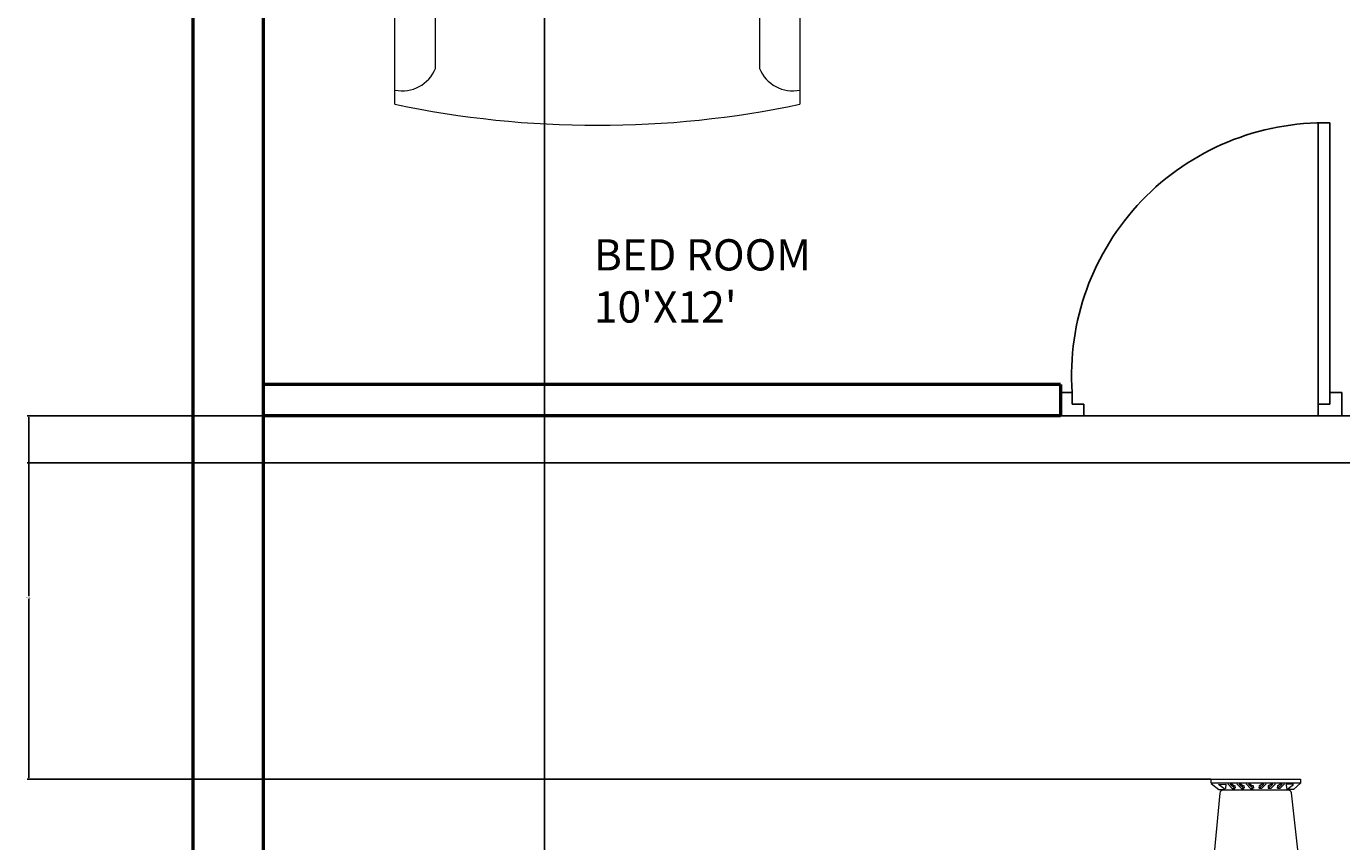
# Model space of a CAD drawing. Units: inches. Extents: x 1798 to 2141, y 1923 to 2386.
# Tile 5 of 9: x 1798 to 1967, y 2177 to 2281. Entities that reach past the tile are written whole.
import ezdxf

# ---------------------------------------------------------------- set-up
doc = ezdxf.new("R2010")
doc.units = ezdxf.units.IN
for name, color, linetype, lineweight in [('A-ANNO-DIMS', 2, 'Continuous', 18), ('A-AREA-IDEN', 7, 'Continuous', 25), ('A-FURN', 8, 'Continuous', 13), ('door', 40, 'Continuous', 25), ('wall', 4, 'Continuous', 50)]:
    doc.layers.add(name, color=color, linetype=linetype, lineweight=lineweight)
doc.styles.get("Standard").update_dxf_attribs({"font": 'arial.ttf'})
doc.dimstyles.get("Standard").update_dxf_attribs({"dimtxt": 0.18, "dimasz": 0.18, "dimexe": 0.18, "dimexo": 0.0625, "dimgap": 0.09, "dimtad": 0, "dimtih": 1, "dimtoh": 1, "dimdec": 4, "dimzin": 0, "dimdsep": 46, "dimtxsty": 'Standard', "dimcen": 0.09, "dimadec": 0, "dimazin": 0, "dimtfac": 1, "dimtdec": 4, "dimtofl": 0, "dimtmove": 0, "dimatfit": 3, "dimfxl": 1, "dimtolj": 1, "dimtzin": 0, "dimarcsym": 0})

# ---------------------------------------------------------------- blocks, each defined once
blk = doc.blocks.new('A$C4F543DC7')
for p, q in [((0.0134, 3.35, -0.1688), (3.3134, 3.35, -0.1688)), ((0.4634, 3.35, -0.1688), (0.0134, 3.35, -0.1688)), ((0.0134, 2.896, -0.1688), (0.0134, 3.35, -0.1688)), ((0.0134, 3.35, -0.1688), (0.0134, 2.896, -0.1688)), ((0.2381, 3.1233, -0.4388), (0.2381, 3.3614, -0.4388)), ((0.4634, 3.35, -0.1688), (0.4634, 0.8, -0.1688)), ((2.8634, 3.35, -0.1688), (0.4634, 3.35, -0.1688)), ((0.4634, 2.896, -0.1688), (0.4634, 3.35, -0.1688)), ((2.8634, 0.8, -0.1688), (2.8634, 3.35, -0.1688)), ((2.8634, 3.35, -0.1688), (3.3134, 3.35, -0.1688)), ((2.8634, 2.896, -0.1688), (2.8634, 3.35, -0.1688)), ((3.0888, 3.1233, -0.4388), (3.0888, 3.3614, -0.4388)), ((3.3134, 3.35, -0.1688), (3.3134, 2.896, -0.1688)), ((3.3134, 3.35, -0.1688), (3.3134, 2.896, -0.1688)), ((1.5354, 3.226, -0.1688), (0.6684, 3.226, -0.1688)), ((2.6644, 3.226, -0.1688), (1.7974, 3.226, -0.1688)), ((0.2381, 3.1233, -0.4388), (0, 3.1233, -0.4388)), ((0.2381, 3.1233, -0.4388), (0.4762, 3.1233, -0.4388)), ((0.2381, 3.1233, -0.4388), (0.2381, 2.8852, -0.4388)), ((0.5684, 3.126, -0.1688), (0.5684, 2.884, -0.1688)), ((1.6354, 2.884, -0.1688), (1.6354, 3.126, -0.1688)), ((1.6974, 3.126, -0.1688), (1.6974, 2.884, -0.1688)), ((2.7644, 2.884, -0.1688), (2.7644, 3.126, -0.1688)), ((3.0888, 3.1233, -0.4388), (2.8507, 3.1233, -0.4388)), ((3.0888, 3.1233, -0.4388), (3.0888, 2.8852, -0.4388)), ((3.0888, 3.1233, -0.4388), (3.3269, 3.1233, -0.4388)), ((0.4634, 2.896, -0.1688), (0.0134, 2.896, -0.1688)), ((0.0134, 2.896, -0.1688), (0.4634, 2.896, -0.1688)), ((0.4634, 0.8, -0.1688), (0.4634, 2.896, -0.1688)), ((2.8634, 2.896, -0.1688), (2.8634, 0.8, -0.1688)), ((3.3134, 2.896, -0.1688), (2.8634, 2.896, -0.1688)), ((3.3134, 2.896, -0.1688), (2.8634, 2.896, -0.1688)), ((0.6684, 2.784, -0.1688), (1.5354, 2.784, -0.1688)), ((1.7974, 2.784, -0.1688), (2.6644, 2.784, -0.1688)), ((1.6534, 2.573, -0.1688), (0.5504, 2.025, -0.1688)), ((0.8414, 1.752, -0.1688), (1.6534, 2.573, -0.1688)), ((2.4814, 1.752, -0.1688), (1.6694, 2.573, -0.1688)), ((1.6694, 2.573, -0.1688), (2.7724, 2.025, -0.1688)), ((0.5504, 2.025, -0.1688), (0.8414, 1.752, -0.1688)), ((2.7724, 2.025, -0.1688), (2.4814, 1.752, -0.1688)), ((2.683, 1.312, -0.1688), (2.7182, 1.3641, -0.1688)), ((0.5369, 1.3267, -0.1688), (0.6088, 1.2835, -0.1688)), ((2.6479, 1.2774, -0.1688), (2.683, 1.312, -0.1688)), ((0.6088, 1.2835, -0.1688), (0.6756, 1.2566, -0.1688)), ((0.6756, 1.2566, -0.1688), (0.7373, 1.2428, -0.1688)), ((0.7373, 1.2428, -0.1688), (0.794, 1.239, -0.1688)), ((0.794, 1.239, -0.1688), (0.8457, 1.242, -0.1688)), ((0.8457, 1.242, -0.1688), (0.8925, 1.2489, -0.1688)), ((0.8925, 1.2489, -0.1688), (0.9345, 1.2564, -0.1688)), ((0.9345, 1.2564, -0.1688), (0.9718, 1.2615, -0.1688)), ((0.9718, 1.2615, -0.1688), (1.0044, 1.2617, -0.1688)), ((1.0044, 1.2617, -0.1688), (1.0334, 1.2578, -0.1688)), ((1.0334, 1.2578, -0.1688), (1.0597, 1.2509, -0.1688)), ((1.0597, 1.2509, -0.1688), (1.0842, 1.2424, -0.1688)), ((1.0842, 1.2424, -0.1688), (1.1081, 1.2336, -0.1688)), ((1.2498, 1.2264, -0.1688), (1.2852, 1.2347, -0.1688)), ((1.2852, 1.2347, -0.1688), (1.3218, 1.2441, -0.1688)), ((1.3218, 1.2441, -0.1688), (1.3591, 1.2533, -0.1688)), ((1.3591, 1.2533, -0.1688), (1.3963, 1.2612, -0.1688)), ((1.3963, 1.2612, -0.1688), (1.4328, 1.2664, -0.1688)), ((1.4328, 1.2664, -0.1688), (1.4679, 1.2677, -0.1688)), ((1.4679, 1.2677, -0.1688), (1.501, 1.2643, -0.1688)), ((1.501, 1.2643, -0.1688), (1.5324, 1.257, -0.1688)), ((1.5324, 1.257, -0.1688), (1.5624, 1.2473, -0.1688)), ((1.5624, 1.2473, -0.1688), (1.5915, 1.2365, -0.1688)), ((1.5915, 1.2365, -0.1688), (1.6199, 1.2259, -0.1688)), ((1.7955, 1.2301, -0.1688), (1.8258, 1.2417, -0.1688)), ((1.8258, 1.2417, -0.1688), (1.8557, 1.2531, -0.1688)), ((1.8557, 1.2531, -0.1688), (1.8849, 1.263, -0.1688)), ((1.8849, 1.263, -0.1688), (1.913, 1.2698, -0.1688)), ((1.913, 1.2698, -0.1688), (1.9397, 1.2722, -0.1688)), ((1.9397, 1.2722, -0.1688), (1.9649, 1.2692, -0.1688)), ((1.9649, 1.2692, -0.1688), (1.989, 1.2617, -0.1688)), ((1.989, 1.2617, -0.1688), (2.0124, 1.2512, -0.1688)), ((2.0124, 1.2512, -0.1688), (2.0359, 1.2391, -0.1688)), ((2.0359, 1.2391, -0.1688), (2.0599, 1.2269, -0.1688)), ((2.2791, 1.2279, -0.1688), (2.3173, 1.2378, -0.1688)), ((2.3173, 1.2378, -0.1688), (2.3558, 1.2465, -0.1688)), ((2.3558, 1.2465, -0.1688), (2.3944, 1.2527, -0.1688)), ((2.3944, 1.2527, -0.1688), (2.4325, 1.255, -0.1688)), ((2.4325, 1.255, -0.1688), (2.4698, 1.2529, -0.1688)), ((2.4698, 1.2529, -0.1688), (2.5064, 1.2488, -0.1688)), ((2.5064, 1.2488, -0.1688), (2.5423, 1.2459, -0.1688)), ((2.5423, 1.2459, -0.1688), (2.5777, 1.2476, -0.1688)), ((2.5777, 1.2476, -0.1688), (2.6129, 1.257, -0.1688)), ((2.6129, 1.257, -0.1688), (2.6479, 1.2774, -0.1688)), ((0.6067, 1.1458, -0.1688), (0.6743, 1.1706, -0.1688)), ((0.6743, 1.1706, -0.1688), (0.7364, 1.1825, -0.1688)), ((0.7364, 1.1825, -0.1688), (0.7931, 1.1846, -0.1688)), ((0.7931, 1.1846, -0.1688), (0.8447, 1.1799, -0.1688)), ((0.8447, 1.1799, -0.1688), (0.8913, 1.1716, -0.1688)), ((0.8913, 1.1716, -0.1688), (0.9331, 1.1628, -0.1688)), ((1.0583, 1.1642, -0.1688), (1.0831, 1.172, -0.1688)), ((1.0831, 1.172, -0.1688), (1.1072, 1.18, -0.1688)), ((1.1072, 1.18, -0.1688), (1.1316, 1.1872, -0.1688)), ((1.1081, 1.2336, -0.1688), (1.1322, 1.2257, -0.1688)), ((1.1316, 1.1872, -0.1688), (1.1573, 1.192, -0.1688)), ((1.1322, 1.2257, -0.1688), (1.1577, 1.2201, -0.1688)), ((1.1573, 1.192, -0.1688), (1.1851, 1.1932, -0.1688)), ((1.1577, 1.2201, -0.1688), (1.1855, 1.218, -0.1688)), ((1.1851, 1.1932, -0.1688), (1.2158, 1.1898, -0.1688)), ((1.1855, 1.218, -0.1688), (1.2163, 1.2204, -0.1688)), ((1.2158, 1.1898, -0.1688), (1.2491, 1.1828, -0.1688)), ((1.2163, 1.2204, -0.1688), (1.2498, 1.2264, -0.1688)), ((1.2491, 1.1828, -0.1688), (1.2842, 1.1734, -0.1688)), ((1.2842, 1.1734, -0.1688), (1.3206, 1.1629, -0.1688)), ((1.5903, 1.1619, -0.1688), (1.6191, 1.1716, -0.1688)), ((1.6191, 1.1716, -0.1688), (1.6475, 1.1797, -0.1688)), ((1.6199, 1.2259, -0.1688), (1.6481, 1.2169, -0.1688)), ((1.6475, 1.1797, -0.1688), (1.676, 1.1849, -0.1688)), ((1.6481, 1.2169, -0.1688), (1.6765, 1.2108, -0.1688)), ((1.676, 1.1849, -0.1688), (1.7049, 1.1858, -0.1688)), ((1.6765, 1.2108, -0.1688), (1.7053, 1.209, -0.1688)), ((1.7049, 1.1858, -0.1688), (1.7344, 1.1816, -0.1688)), ((1.7053, 1.209, -0.1688), (1.7349, 1.2124, -0.1688)), ((1.7344, 1.1816, -0.1688), (1.7643, 1.1731, -0.1688)), ((1.7349, 1.2124, -0.1688), (1.7651, 1.2199, -0.1688)), ((1.7643, 1.1731, -0.1688), (1.7944, 1.1619, -0.1688)), ((1.7651, 1.2199, -0.1688), (1.7955, 1.2301, -0.1688)), ((2.0599, 1.2269, -0.1688), (2.0849, 1.216, -0.1688)), ((2.0842, 1.167, -0.1688), (2.1112, 1.1743, -0.1688)), ((2.0849, 1.216, -0.1688), (2.1117, 1.2077, -0.1688)), ((2.1112, 1.1743, -0.1688), (2.1403, 1.1775, -0.1688)), ((2.1117, 1.2077, -0.1688), (2.1407, 1.2037, -0.1688)), ((2.1403, 1.1775, -0.1688), (2.1718, 1.1755, -0.1688)), ((2.1407, 1.2037, -0.1688), (2.1723, 1.2047, -0.1688)), ((2.1718, 1.1755, -0.1688), (2.2056, 1.1691, -0.1688)), ((2.1723, 1.2047, -0.1688), (2.2062, 1.21, -0.1688)), ((2.2062, 1.21, -0.1688), (2.242, 1.2182, -0.1688)), ((2.242, 1.2182, -0.1688), (2.2791, 1.2279, -0.1688)), ((0.5334, 1.105, -0.1688), (0.6067, 1.1458, -0.1688)), ((0.9331, 1.1628, -0.1688), (0.9701, 1.1565, -0.1688)), ((0.9701, 1.1565, -0.1688), (1.0027, 1.1552, -0.1688)), ((1.0027, 1.1552, -0.1688), (1.0318, 1.1582, -0.1688)), ((1.0318, 1.1582, -0.1688), (1.0583, 1.1642, -0.1688)), ((1.3206, 1.1629, -0.1688), (1.3575, 1.1524, -0.1688)), ((1.3575, 1.1524, -0.1688), (1.3945, 1.1434, -0.1688)), ((1.3945, 1.1434, -0.1688), (1.4308, 1.1371, -0.1688)), ((1.4308, 1.1371, -0.1688), (1.4658, 1.1347, -0.1688)), ((1.4658, 1.1347, -0.1688), (1.499, 1.137, -0.1688)), ((1.499, 1.137, -0.1688), (1.5306, 1.1433, -0.1688)), ((1.5306, 1.1433, -0.1688), (1.5609, 1.152, -0.1688)), ((1.5609, 1.152, -0.1688), (1.5903, 1.1619, -0.1688)), ((1.7944, 1.1619, -0.1688), (1.8244, 1.1494, -0.1688)), ((1.8244, 1.1494, -0.1688), (1.8539, 1.137, -0.1688)), ((1.8539, 1.137, -0.1688), (1.8827, 1.1263, -0.1688)), ((1.8827, 1.1263, -0.1688), (1.9106, 1.1186, -0.1688)), ((1.9106, 1.1186, -0.1688), (1.9373, 1.1153, -0.1688)), ((1.9373, 1.1153, -0.1688), (1.9625, 1.1176, -0.1688)), ((1.9625, 1.1176, -0.1688), (1.9868, 1.1243, -0.1688)), ((1.9868, 1.1243, -0.1688), (2.0106, 1.134, -0.1688)), ((2.0106, 1.134, -0.1688), (2.0344, 1.1454, -0.1688)), ((2.0344, 1.1454, -0.1688), (2.0588, 1.1568, -0.1688)), ((2.0588, 1.1568, -0.1688), (2.0842, 1.167, -0.1688)), ((2.2056, 1.1691, -0.1688), (2.2411, 1.1598, -0.1688)), ((2.2411, 1.1598, -0.1688), (2.2779, 1.1489, -0.1688)), ((2.2779, 1.1489, -0.1688), (2.3157, 1.1379, -0.1688)), ((2.3157, 1.1379, -0.1688), (2.354, 1.1279, -0.1688)), ((2.354, 1.1279, -0.1688), (2.3923, 1.1205, -0.1688)), ((2.3923, 1.1205, -0.1688), (2.4304, 1.117, -0.1688)), ((2.4304, 1.117, -0.1688), (2.4677, 1.118, -0.1688)), ((2.4677, 1.118, -0.1688), (2.5043, 1.1209, -0.1688)), ((2.5043, 1.1209, -0.1688), (2.5403, 1.1226, -0.1688)), ((2.5403, 1.1226, -0.1688), (2.5757, 1.1199, -0.1688)), ((2.5757, 1.1199, -0.1688), (2.6106, 1.1094, -0.1688)), ((2.6106, 1.1094, -0.1688), (2.645, 1.0879, -0.1688)), ((2.645, 1.0879, -0.1688), (2.6789, 1.0522, -0.1688)), ((2.6789, 1.0522, -0.1688), (2.7124, 0.999, -0.1688)), ((0.4634, 0.85, -0.1688), (2.8634, 0.85, -0.1688)), ((0.4634, 0.8, -0.1688), (2.8634, 0.8, -0.1688)), ((0.6634, 0.8, -0.1688), (0.4634, 0.8, -0.1688)), ((0.6634, 0.8, -0.1688), (2.6634, 0.8, -0.1688)), ((0.6634, 0.104, -0.1688), (0.6634, 0.8, -0.1688)), ((0.6634, 0.104, -0.1688), (0.6634, 0.8, -0.1688)), ((0.8634, 0.281, -0.1688), (0.8634, 0.8, -0.1688)), ((2.4634, 0.8, -0.1688), (2.4634, 0.281, -0.1688)), ((2.8634, 0.8, -0.1688), (2.6634, 0.8, -0.1688)), ((2.6634, 0.8, -0.1688), (2.6634, 0.104, -0.1688)), ((2.6634, 0.8, -0.1688), (2.6634, 0.104, -0.1688))]:
    blk.add_line(p, q)
for centre, radius in [((0.2381, 3.1233, -0.4388), 0.139), ((3.0888, 3.1233, -0.4388), 0.139), ((0.2381, 3.1233, -0.4388), 0.075), ((3.0888, 3.1233, -0.4388), 0.075)]:
    blk.add_circle(centre, radius)
for centre, radius, start, end in [((0.6684, 3.126, -0.1688), 0.1, 90, 180), ((1.5354, 3.126, -0.1688), 0.1, 0, 90), ((1.7974, 3.126, -0.1688), 0.1, 90, 180), ((2.6644, 3.126, -0.1688), 0.1, 0, 90), ((0.6684, 2.884, -0.1688), 0.1, 180, 270), ((1.5354, 2.884, -0.1688), 0.1, 270, 0), ((1.7974, 2.884, -0.1688), 0.1, 180, 270), ((2.6644, 2.884, -0.1688), 0.1, 270, 0), ((0.6994, 0.3472, -0.1688), 0.1769, 258.2616, 338.03196), ((2.6275, 0.3472, -0.1688), 0.1769, 201.96804, 281.7384), ((1.6634, 4.8597, -0.1688), 4.8597, 258.12517, 281.87483), ((1.6634, 4.8597, -0.1688), 4.8597, 258.12517, 281.87483)]:
    blk.add_arc(centre, radius, start, end)
blk = doc.blocks.new('A$C45501D90')
for p, q in [((-242.2, 1133.5), (224, 1133.5)), ((-242.2, 1112.8), (-242.2, 1133.5)), ((224, 1112.8), (-242.2, 1112.8)), ((-242.2, 1111.2), (-202.3, 1079.2)), ((-203.9, 1106.4), (-165.6, 1108)), ((-168.8, 1080.8), (-203.9, 1106.4)), ((-165.6, 1108), (-167.2, 1085.6)), ((-156, 1109.6), (-132, 1085.6)), ((-119.3, 1085.6), (-143.2, 1108)), ((-143.2, 1108), (-133.6, 1108)), ((-133.6, 1108), (-122.5, 1098.4)), ((-122.5, 1098.4), (-119.3, 1101.6)), ((-119.3, 1101.6), (-117.7, 1087.2)), ((-108.1, 1109.6), (-84.1, 1085.6)), ((-71.4, 1085.6), (-95.3, 1108)), ((-95.3, 1108), (-85.7, 1108)), ((-85.7, 1108), (-74.6, 1098.4)), ((-74.6, 1098.4), (-71.4, 1101.6)), ((-71.4, 1101.6), (-69.8, 1087.2)), ((-60.2, 1109.6), (-36.2, 1085.6)), ((-23.5, 1085.6), (-47.4, 1108)), ((-47.4, 1108), (-37.8, 1108)), ((-37.8, 1108), (-26.7, 1098.4)), ((-26.7, 1098.4), (-23.5, 1101.6)), ((-23.5, 1101.6), (-21.9, 1087.2)), ((8.5, 1101.6), (6.9, 1087.2)), ((8.5, 1085.6), (32.4, 1108)), ((11.6, 1098.4), (8.5, 1101.6)), ((22.8, 1108), (11.6, 1098.4)), ((45.2, 1109.6), (21.2, 1085.6)), ((32.4, 1108), (22.8, 1108)), ((56.3, 1101.6), (54.8, 1087.2)), ((56.3, 1085.6), (80.3, 1108)), ((59.5, 1098.4), (56.3, 1101.6)), ((70.7, 1108), (59.5, 1098.4)), ((93.1, 1109.6), (69.1, 1085.6)), ((80.3, 1108), (70.7, 1108)), ((104.2, 1101.6), (102.6, 1087.2)), ((104.2, 1085.6), (128.2, 1108)), ((107.4, 1098.4), (104.2, 1101.6)), ((118.6, 1108), (107.4, 1098.4)), ((141, 1109.6), (117, 1085.6)), ((128.2, 1108), (118.6, 1108)), ((188.9, 1106.4), (150.5, 1108)), ((150.5, 1108), (152.1, 1085.6)), ((153.7, 1080.8), (188.9, 1106.4)), ((224, 1112.8), (187.3, 1079.2)), ((224, 1133.5), (224, 1112.8)), ((-197.3, 1061.6), (-238.9, 627.6)), ((-202.3, 1079.2), (-168.8, 1080.8)), ((161.8, 1076.1), (-181.4, 1076.1)), ((-132, 1085.6), (-119.3, 1085.6)), ((-84.1, 1085.6), (-71.4, 1085.6)), ((-36.2, 1085.6), (-23.5, 1085.6)), ((21.2, 1085.6), (8.5, 1085.6)), ((69.1, 1085.6), (56.3, 1085.6)), ((117, 1085.6), (104.2, 1085.6)), ((187.3, 1079.2), (153.7, 1080.8)), ((225.2, 627.8), (177.6, 1061.8)), ((-1102.7, 357), (-869.7, 760.7)), ((-869.7, 760.7), (-851.7, 750.4)), ((841.2, 765.3), (833.5, 714.8)), ((842.6, 766.1), (860.5, 776.5)), ((1075.7, 362.4), (842.6, 766.1)), ((860.5, 776.5), (1093.6, 372.8)), ((-851.7, 750.4), (-1084.8, 346.6)), ((-863.7, 716.7), (-884.3, 684.4)), ((-859.2, 673.6), (-863.7, 716.7)), ((-841, 701.8), (-859.2, 673.6)), ((-848.7, 752.3), (-841, 701.8)), ((820.7, 701.7), (424.1, 520.7)), ((833.5, 714.8), (851.7, 686.6)), ((1012.8, 397.9), (841.2, 695.1)), ((851.7, 686.6), (856.2, 729.8)), ((856.2, 729.8), (876.7, 697.4)), ((876.7, 697.4), (856.6, 687.6)), ((882.9, 689.9), (874.2, 657.2)), ((-851, 678.1), (-1022.6, 380.9)), ((-919.4, 623.5), (-924.2, 615.2)), ((-912, 591.6), (-919.4, 623.5)), ((-914.4, 635.4), (-905.6, 602.7)), ((-897.5, 642.2), (-901.9, 641.1)), ((-901.9, 641.1), (-890.2, 632.5)), ((-895.4, 665), (-900.2, 656.7)), ((-900.2, 656.7), (-897.5, 642.2)), ((-888.1, 633.1), (-895.4, 665)), ((-890.4, 676.9), (-881.7, 644.2)), ((-881.7, 644.2), (-888.1, 633.1)), ((-884.3, 684.4), (-864.1, 674.6)), ((-431.1, 509), (-830.8, 684.8)), ((874.2, 657.2), (880.6, 646.1)), ((880.6, 646.1), (887.9, 678)), ((894.4, 654.1), (882.7, 645.5)), ((887.9, 678), (892.7, 669.7)), ((892.7, 669.7), (890, 655.2)), ((890, 655.2), (894.4, 654.1)), ((906.9, 648.4), (898.1, 615.7)), ((904.5, 604.6), (911.9, 636.5)), ((911.9, 636.5), (916.7, 628.2)), ((916.7, 628.2), (914, 613.8)), ((-945.4, 559.3), (-949.8, 558.1)), ((-949.8, 558.1), (-938.1, 549.6)), ((-943.3, 582), (-948.1, 573.8)), ((-948.1, 573.8), (-945.4, 559.3)), ((-936, 550.1), (-943.3, 582)), ((-938.3, 593.9), (-929.6, 561.2)), ((-929.6, 561.2), (-936, 550.1)), ((-921.5, 600.8), (-925.8, 599.6)), ((-925.8, 599.6), (-914.2, 591)), ((-924.2, 615.2), (-921.5, 600.8)), ((-905.6, 602.7), (-912, 591.6)), ((-223, 610.1), (209.4, 610.1)), ((898.1, 615.7), (904.5, 604.6)), ((918.3, 612.6), (906.7, 604)), ((914, 613.8), (918.3, 612.6)), ((930.8, 606.9), (922.1, 574.2)), ((922.1, 574.2), (928.4, 563.1)), ((928.4, 563.1), (935.8, 595.1)), ((942.3, 571.1), (930.6, 562.6)), ((935.8, 595.1), (940.6, 586.8)), ((940.6, 586.8), (937.9, 572.3)), ((937.9, 572.3), (942.3, 571.1)), ((-1002.4, 479.7), (-988.5, 484.6)), ((-991, 502.7), (-958.3, 511.4)), ((-988.5, 484.6), (-989.7, 489)), ((-989.7, 489), (-976.5, 483.2)), ((-951.9, 522.5), (-983.2, 512.9)), ((-983.2, 512.9), (-978.5, 521.2)), ((-978.5, 521.2), (-964.6, 526.1)), ((-964.6, 526.1), (-965.7, 530.5)), ((-965.7, 530.5), (-952.5, 524.7)), ((-958.3, 511.4), (-951.9, 522.5)), ((-639.9, 111.9), (-423.7, 486.4)), ((-5.6, 508.7, 90.8), (0.4, 508.7, 90.8)), ((-5.6, 317.7, 90.8), (-5.6, 508.7, 90.8)), ((0.4, 508.7, 90.8), (0.4, 317.7, 90.8)), ((5.8, 317.7, 90.8), (5.8, 508.7, 90.8)), ((5.8, 508.7, 90.8), (11.8, 508.7, 90.8)), ((11.8, 508.7, 90.8), (11.8, 317.7, 90.8)), ((416.9, 498.2), (633.1, 123.7)), ((950.8, 524.4), (944.4, 535.5)), ((944.4, 535.5), (975.7, 525.9)), ((958.2, 543.5), (945, 537.7)), ((983.5, 515.7), (950.8, 524.4)), ((957.1, 539.1), (958.2, 543.5)), ((970.9, 534.2), (957.1, 539.1)), ((968.4, 494), (999.7, 484.4)), ((974.7, 483), (968.4, 494)), ((982.2, 502), (968.9, 496.2)), ((975.7, 525.9), (970.9, 534.2)), ((1007.4, 474.2), (974.7, 483)), ((981, 497.6), (982.2, 502)), ((994.9, 492.7), (981, 497.6)), ((999.7, 484.4), (994.9, 492.7)), ((-1038.9, 419.7), (-1006.2, 428.5)), ((-999.8, 439.5), (-1031.1, 430)), ((-1031.1, 430), (-1026.3, 438.3)), ((-1026.3, 438.3), (-1012.5, 443.1)), ((-1015, 461.2), (-982.3, 469.9)), ((-1012.5, 443.1), (-1013.6, 447.5)), ((-1013.6, 447.5), (-1000.4, 441.7)), ((-975.9, 481), (-1007.2, 471.4)), ((-1007.2, 471.4), (-1002.4, 479.7)), ((-1006.2, 428.5), (-999.8, 439.5)), ((-982.3, 469.9), (-975.9, 481)), ((998.7, 441.5), (992.3, 452.5)), ((992.3, 452.5), (1023.6, 443)), ((1006.1, 460.5), (992.9, 454.7)), ((1031.4, 432.7), (998.7, 441.5)), ((1005, 456.2), (1006.1, 460.5)), ((1018.8, 451.3), (1005, 456.2)), ((1034.8, 423.6), (1016.3, 411.1)), ((1023.6, 443), (1018.8, 451.3)), ((1052.6, 389.6), (1034.8, 423.6)), ((-1084.8, 346.6), (-1102.7, 357)), ((-1083.4, 345.8), (-1035.8, 364.4)), ((-1060.1, 376.6), (-1042.3, 410.6)), ((-1020.4, 394.3), (-1060.1, 376.6)), ((-1042.3, 410.6), (-1023.8, 398.1)), ((-1035.8, 364.4), (-1020.4, 394.3)), ((-1018, 360), (-663, 106.9)), ((-22.3, 329.1, 90.8), (-22.3, 344.6, 90.8)), ((-22.3, 344.6, 90.8), (-5.6, 344.6, 90.8)), ((0.4, 344.6, 90.8), (5.8, 344.6, 90.8)), ((11.8, 344.6, 90.8), (27.3, 344.6, 90.8)), ((27.3, 344.6, 90.8), (27.3, 329.1, 90.8)), ((656.3, 118.9), (1008.4, 377.1)), ((1028.3, 377.5), (1012.9, 407.3)), ((1012.9, 407.3), (1052.6, 389.6)), ((1075.9, 358.8), (1028.3, 377.5)), ((1093.6, 372.8), (1075.7, 362.4)), ((-430.6, 275.2, 90.8), (-427.6, 280.3, 90.8)), ((-427.6, 280.3, 90.8), (-262.3, 184.9, 90.8)), ((-175.3, 276.1, 90.8), (-104.8, 293.2, 90.8)), ((-103.3, 252.4, 90.8), (-175.3, 276.1, 90.8)), ((-104.8, 293.2, 90.8), (-85.5, 278.4, 90.8)), ((-85.5, 278.4, 90.8), (-52.1, 293.9, 90.8)), ((9.5, 276.1, 90.8), (-59.5, 246.5, 90.8)), ((-52.1, 293.9, 90.8), (9.5, 276.1, 90.8)), ((-5.6, 329.1, 90.8), (-22.3, 329.1, 90.8)), ((0.4, 317.7, 90.8), (-5.6, 317.7, 90.8)), ((5.8, 329.1, 90.8), (0.4, 329.1, 90.8)), ((11.8, 317.7, 90.8), (5.8, 317.7, 90.8)), ((27.3, 329.1, 90.8), (11.8, 329.1, 90.8)), ((134.3, 288, 90.8), (184.3, 235.5, 90.8)), ((149.7, 213.9, 90.8), (134.3, 288, 90.8)), ((-436.3, 265.3, 90.8), (-433.3, 270.5, 90.8)), ((-270.9, 169.9, 90.8), (-436.3, 265.3, 90.8)), ((-433.3, 270.5, 90.8), (-267.9, 175, 90.8)), ((-265.2, 179.7, 90.8), (-430.6, 275.2, 90.8)), ((-285.5, 198.3, 90.8), (-277.8, 211.7, 90.8)), ((-277.8, 211.7, 90.8), (-264.3, 204, 90.8)), ((-59.5, 246.5, 90.8), (-103.3, 252.4, 90.8)), ((166.5, 173, 90.8), (149.7, 213.9, 90.8)), ((184.3, 235.5, 90.8), (181.1, 211.4, 90.8)), ((181.1, 211.4, 90.8), (211.3, 190.3, 90.8)), ((255.2, 161.9, 90.8), (420.6, 257.3, 90.8)), ((423.5, 252.2, 90.8), (258.2, 156.7, 90.8)), ((260.9, 152, 90.8), (426.2, 247.5, 90.8)), ((429.2, 242.3, 90.8), (263.8, 146.9, 90.8)), ((420.6, 257.3, 90.8), (423.5, 252.2, 90.8)), ((426.2, 247.5, 90.8), (429.2, 242.3, 90.8)), ((-302.5, 168.8, 90.8), (-294.2, 183.3, 90.8)), ((-289.1, 161.1, 90.8), (-302.5, 168.8, 90.8)), ((-291.2, 188.5, 90.8), (-288.5, 193.1, 90.8)), ((-280.7, 175.5, 90.8), (-289.1, 161.1, 90.8)), ((-275.1, 185.4, 90.8), (-277.8, 180.7, 90.8)), ((-273.6, 117.6, 90.8), (-227.4, 162.1, 90.8)), ((-264.3, 204, 90.8), (-272.1, 190.5, 90.8)), ((-267.9, 175, 90.8), (-270.9, 169.9, 90.8)), ((-262.3, 184.9, 90.8), (-265.2, 179.7, 90.8)), ((-227.4, 162.1, 90.8), (-236.2, 87.5, 90.8)), ((226.7, 128.1, 90.8), (166.5, 173, 90.8)), ((211.3, 190.3, 90.8), (226.7, 128.1, 90.8)), ((258.2, 156.7, 90.8), (255.2, 161.9, 90.8)), ((256.6, 182, 90.8), (270.1, 189.8, 90.8)), ((265, 167.5, 90.8), (256.6, 182, 90.8)), ((263.8, 146.9, 90.8), (260.9, 152, 90.8)), ((270.7, 157.7, 90.8), (268, 162.4, 90.8)), ((270.1, 189.8, 90.8), (278.4, 175.3, 90.8)), ((281.4, 139.1, 90.8), (273.7, 152.5, 90.8)), ((281.4, 170.1, 90.8), (284.1, 165.5, 90.8)), ((294.9, 146.8, 90.8), (281.4, 139.1, 90.8)), ((287.1, 160.3, 90.8), (294.9, 146.8, 90.8)), ((-319.8, 2.1, 90.8), (-299.3, 71.7, 90.8)), ((-299.3, 71.7, 90.8), (-276.8, 80.9, 90.8)), ((-276.8, 80.9, 90.8), (-273.6, 117.6, 90.8)), ((-236.2, 87.5, 90.8), (-263.2, 52.5, 90.8)), ((-263.2, 52.5, 90.8), (-319.8, 2.1, 90.8)), ((242.9, -24.6, 90.8), (299.4, 25.9, 90.8)), ((299.4, 25.9, 90.8), (278.9, -43.7, 90.8)), ((207, -134.1, 90.8), (215.8, -59.5, 90.8)), ((215.8, -59.5, 90.8), (242.9, -24.6, 90.8)), ((256.4, -53, 90.8), (253.2, -89.7, 90.8)), ((278.9, -43.7, 90.8), (256.4, -53, 90.8)), ((-656.3, -118.9), (-1008.4, -377.1)), ((-416.9, -498.2), (-633.1, -123.7)), ((-449.6, -214.4, 90.8), (-284.2, -118.9, 90.8)), ((-281.2, -124.1, 90.8), (-446.6, -219.5, 90.8)), ((-443.9, -224.2, 90.8), (-278.5, -128.7, 90.8)), ((-275.5, -133.9, 90.8), (-440.9, -229.4, 90.8)), ((-315.2, -118.9, 90.8), (-301.8, -111.1, 90.8)), ((-307.5, -132.3, 90.8), (-315.2, -118.9, 90.8)), ((-301.8, -142.1, 90.8), (-304.5, -137.5, 90.8)), ((-301.8, -111.1, 90.8), (-294, -124.6, 90.8)), ((-291, -129.7, 90.8), (-288.3, -134.4, 90.8)), ((-284.2, -118.9, 90.8), (-281.2, -124.1, 90.8)), ((-278.5, -128.7, 90.8), (-275.5, -133.9, 90.8)), ((-247, -100.1, 90.8), (-186.8, -145, 90.8)), ((-231.7, -162.3, 90.8), (-247, -100.1, 90.8)), ((253.2, -89.7, 90.8), (207, -134.1, 90.8)), ((260.4, -147.6, 90.8), (268.7, -133.1, 90.8)), ((268.7, -133.1, 90.8), (282.2, -140.8, 90.8)), ((639.9, -111.9), (423.7, -486.4)), ((1018, -360), (663, -106.9)), ((-290.4, -161.8, 90.8), (-298.8, -147.3, 90.8)), ((-277, -154, 90.8), (-290.4, -161.8, 90.8)), ((-285.4, -139.5, 90.8), (-277, -154, 90.8)), ((-201.5, -183.4, 90.8), (-231.7, -162.3, 90.8)), ((-204.7, -207.6, 90.8), (-201.5, -183.4, 90.8)), ((-186.8, -145, 90.8), (-170.1, -185.9, 90.8)), ((-170.1, -185.9, 90.8), (-154.7, -260.1, 90.8)), ((241.9, -156.9, 90.8), (244.9, -151.7, 90.8)), ((407.3, -252.4, 90.8), (241.9, -156.9, 90.8)), ((244, -176, 90.8), (251.7, -162.5, 90.8)), ((257.4, -183.7, 90.8), (244, -176, 90.8)), ((244.9, -151.7, 90.8), (410.3, -247.2, 90.8)), ((247.6, -147.1, 90.8), (250.6, -141.9, 90.8)), ((413, -242.5, 90.8), (247.6, -147.1, 90.8)), ((250.6, -141.9, 90.8), (415.9, -237.4, 90.8)), ((254.7, -157.4, 90.8), (257.4, -152.7, 90.8)), ((265.2, -170.3, 90.8), (257.4, -183.7, 90.8)), ((270.8, -160.5, 90.8), (268.1, -165.1, 90.8)), ((282.2, -140.8, 90.8), (273.8, -155.3, 90.8)), ((-446.6, -219.5, 90.8), (-449.6, -214.4, 90.8)), ((-440.9, -229.4, 90.8), (-443.9, -224.2, 90.8)), ((-154.7, -260.1, 90.8), (-204.7, -207.6, 90.8)), ((-29.8, -248.2, 90.8), (39.2, -218.5, 90.8)), ((31.8, -266, 90.8), (-29.8, -248.2, 90.8)), ((65.2, -250.4, 90.8), (31.8, -266, 90.8)), ((39.2, -218.5, 90.8), (83, -224.4, 90.8)), ((84.4, -265.2, 90.8), (65.2, -250.4, 90.8)), ((83, -224.4, 90.8), (154.9, -248.2, 90.8)), ((154.9, -248.2, 90.8), (84.4, -265.2, 90.8)), ((410.3, -247.2, 90.8), (407.3, -252.4, 90.8)), ((415.9, -237.4, 90.8), (413, -242.5, 90.8)), ((-47.6, -316.6, 90.8), (-47.6, -301.1, 90.8)), ((-47.6, -301.1, 90.8), (-32.1, -301.1, 90.8)), ((-32.1, -316.6, 90.8), (-47.6, -316.6, 90.8)), ((-32.1, -480.7, 90.8), (-32.1, -289.8, 90.8)), ((-32.1, -289.8, 90.8), (-26.1, -289.8, 90.8)), ((-26.1, -289.8, 90.8), (-26.1, -480.7, 90.8)), ((-26.1, -301.1, 90.8), (-20.8, -301.1, 90.8)), ((-20.8, -316.6, 90.8), (-26.1, -316.6, 90.8)), ((-20.8, -480.7, 90.8), (-20.8, -289.8, 90.8)), ((-20.8, -289.8, 90.8), (-14.8, -289.8, 90.8)), ((-14.8, -289.8, 90.8), (-14.8, -480.7, 90.8)), ((-14.8, -301.1, 90.8), (1.9, -301.1, 90.8)), ((1.9, -316.6, 90.8), (-14.8, -316.6, 90.8)), ((1.9, -301.1, 90.8), (1.9, -316.6, 90.8)), ((-1093.6, -372.8), (-1075.7, -362.4)), ((-860.5, -776.5), (-1093.6, -372.8)), ((-1075.9, -358.8), (-1028.3, -377.5)), ((-1075.7, -362.4), (-842.6, -766.1)), ((-1052.6, -389.6), (-1034.8, -423.6)), ((-1012.9, -407.3), (-1052.6, -389.6)), ((-1034.8, -423.6), (-1016.3, -411.1)), ((-1028.3, -377.5), (-1012.9, -407.3)), ((-1012.8, -397.9), (-841.2, -695.1)), ((851, -678.1), (1022.6, -380.9)), ((851.7, -750.4), (1084.8, -346.6)), ((1102.7, -357), (869.7, -760.7)), ((1035.8, -364.4), (1020.4, -394.3)), ((1020.4, -394.3), (1060.1, -376.6)), ((1042.3, -410.6), (1023.8, -398.1)), ((1083.4, -345.8), (1035.8, -364.4)), ((1060.1, -376.6), (1042.3, -410.6)), ((1084.8, -346.6), (1102.7, -357)), ((-1031.4, -432.7), (-998.7, -441.5)), ((-1023.6, -443), (-1018.8, -451.3)), ((-992.3, -452.5), (-1023.6, -443)), ((-1018.8, -451.3), (-1005, -456.2)), ((-1007.4, -474.2), (-974.7, -483)), ((-1006.1, -460.5), (-992.9, -454.7)), ((-1005, -456.2), (-1006.1, -460.5)), ((-998.7, -441.5), (-992.3, -452.5)), ((-26.1, -480.7, 90.8), (-32.1, -480.7, 90.8)), ((-14.8, -480.7, 90.8), (-20.8, -480.7, 90.8)), ((982.3, -469.9), (975.9, -481)), ((975.9, -481), (1007.2, -471.4)), ((1015, -461.2), (982.3, -469.9)), ((1002.4, -479.7), (988.5, -484.6)), ((1006.2, -428.5), (999.8, -439.5)), ((999.8, -439.5), (1031.1, -430)), ((1013.6, -447.5), (1000.4, -441.7)), ((1007.2, -471.4), (1002.4, -479.7)), ((1038.9, -419.7), (1006.2, -428.5)), ((1026.3, -438.3), (1012.5, -443.1)), ((1012.5, -443.1), (1013.6, -447.5)), ((1031.1, -430), (1026.3, -438.3)), ((-968.4, -494), (-999.7, -484.4)), ((-999.7, -484.4), (-994.9, -492.7)), ((-994.9, -492.7), (-981, -497.6)), ((-983.5, -515.7), (-950.8, -524.4)), ((-982.2, -502), (-968.9, -496.2)), ((-981, -497.6), (-982.2, -502)), ((-944.4, -535.5), (-975.7, -525.9)), ((-975.7, -525.9), (-970.9, -534.2)), ((-974.7, -483), (-968.4, -494)), ((-970.9, -534.2), (-957.1, -539.1)), ((-958.2, -543.5), (-945, -537.7)), ((-957.1, -539.1), (-958.2, -543.5)), ((-950.8, -524.4), (-944.4, -535.5)), ((-820.7, -701.7), (-424.1, -520.7)), ((431.1, -509), (830.8, -684.8)), ((929.6, -561.2), (936, -550.1)), ((936, -550.1), (943.3, -582)), ((949.8, -558.1), (938.1, -549.6)), ((958.3, -511.4), (951.9, -522.5)), ((951.9, -522.5), (983.2, -512.9)), ((965.7, -530.5), (952.5, -524.7)), ((991, -502.7), (958.3, -511.4)), ((978.5, -521.2), (964.6, -526.1)), ((964.6, -526.1), (965.7, -530.5)), ((989.7, -489), (976.5, -483.2)), ((983.2, -512.9), (978.5, -521.2)), ((988.5, -484.6), (989.7, -489)), ((-942.3, -571.1), (-930.6, -562.6)), ((-937.9, -572.3), (-942.3, -571.1)), ((-940.6, -586.8), (-937.9, -572.3)), ((-935.8, -595.1), (-940.6, -586.8)), ((-928.4, -563.1), (-935.8, -595.1)), ((-930.8, -606.9), (-922.1, -574.2)), ((-922.1, -574.2), (-928.4, -563.1)), ((-918.3, -612.6), (-906.7, -604)), ((-914, -613.8), (-918.3, -612.6)), ((-916.7, -628.2), (-914, -613.8)), ((-904.5, -604.6), (-911.9, -636.5)), ((-906.9, -648.4), (-898.1, -615.7)), ((-898.1, -615.7), (-904.5, -604.6)), ((218.9, -611.6), (-213.5, -611.6)), ((223, -610.1), (-209.4, -610.1)), ((905.6, -602.7), (912, -591.6)), ((914.4, -635.4), (905.6, -602.7)), ((912, -591.6), (919.4, -623.5)), ((925.8, -599.6), (914.2, -591)), ((919.4, -623.5), (924.2, -615.2)), ((921.5, -600.8), (925.8, -599.6)), ((924.2, -615.2), (921.5, -600.8)), ((938.3, -593.9), (929.6, -561.2)), ((943.3, -582), (948.1, -573.8)), ((945.4, -559.3), (949.8, -558.1)), ((948.1, -573.8), (945.4, -559.3)), ((-911.9, -636.5), (-916.7, -628.2)), ((-894.4, -654.1), (-882.7, -645.5)), ((-890, -655.2), (-894.4, -654.1)), ((-892.7, -669.7), (-890, -655.2)), ((-887.9, -678), (-892.7, -669.7)), ((-880.6, -646.1), (-887.9, -678)), ((-882.9, -689.9), (-874.2, -657.2)), ((-874.2, -657.2), (-880.6, -646.1)), ((-876.7, -697.4), (-856.6, -687.6)), ((-851.7, -686.6), (-856.2, -729.8)), ((-833.5, -714.8), (-851.7, -686.6)), ((-229.3, -629.3), (-181.8, -1063.3)), ((-225.2, -627.8), (-177.6, -1061.8)), ((193.2, -1063.1), (234.8, -629.1)), ((197.3, -1061.6), (238.9, -627.6)), ((841, -701.8), (859.2, -673.6)), ((859.2, -673.6), (863.7, -716.7)), ((863.7, -716.7), (884.3, -684.4)), ((884.3, -684.4), (864.1, -674.6)), ((881.7, -644.2), (888.1, -633.1)), ((890.4, -676.9), (881.7, -644.2)), ((888.1, -633.1), (895.4, -665)), ((901.9, -641.1), (890.2, -632.5)), ((895.4, -665), (900.2, -656.7)), ((897.5, -642.2), (901.9, -641.1)), ((900.2, -656.7), (897.5, -642.2)), ((-856.2, -729.8), (-876.7, -697.4)), ((-841.2, -765.3), (-833.5, -714.8)), ((848.7, -752.3), (841, -701.8)), ((869.7, -760.7), (851.7, -750.4)), ((-842.6, -766.1), (-860.5, -776.5)), ((-231.3, -1112.7), (-191.4, -1080.8)), ((-227.2, -1111.2), (-187.3, -1079.2)), ((-157.9, -1082.4), (-193, -1107.9)), ((-191.4, -1080.8), (-157.9, -1082.4)), ((-153.7, -1080.8), (-188.9, -1106.4)), ((-187.3, -1079.2), (-153.7, -1080.8)), ((-165.9, -1077.6), (177.3, -1077.6)), ((-161.8, -1076.1), (181.4, -1076.1)), ((-154.7, -1109.5), (-156.3, -1087.1)), ((-150.5, -1108), (-152.1, -1085.6)), ((-145.1, -1111.1), (-121.1, -1087.1)), ((-141, -1109.6), (-117, -1085.6)), ((-108.4, -1087.1), (-132.3, -1109.5)), ((-104.2, -1085.6), (-128.2, -1108)), ((-122.7, -1109.5), (-111.6, -1099.9)), ((-121.1, -1087.1), (-108.4, -1087.1)), ((-118.6, -1108), (-107.4, -1098.4)), ((-117, -1085.6), (-104.2, -1085.6)), ((-111.6, -1099.9), (-108.4, -1103.1)), ((-108.4, -1103.1), (-106.8, -1088.7)), ((-107.4, -1098.4), (-104.2, -1101.6)), ((-104.2, -1101.6), (-102.6, -1087.2)), ((-97.2, -1111.1), (-73.2, -1087.1)), ((-93.1, -1109.6), (-69.1, -1085.6)), ((-60.5, -1087.1), (-84.4, -1109.5)), ((-56.3, -1085.6), (-80.3, -1108)), ((-74.8, -1109.5), (-63.7, -1099.9)), ((-73.2, -1087.1), (-60.5, -1087.1)), ((-70.7, -1108), (-59.5, -1098.4)), ((-69.1, -1085.6), (-56.3, -1085.6)), ((-63.7, -1099.9), (-60.5, -1103.1)), ((-60.5, -1103.1), (-58.9, -1088.7)), ((-59.5, -1098.4), (-56.3, -1101.6)), ((-56.3, -1101.6), (-54.8, -1087.2)), ((-49.3, -1111.1), (-25.3, -1087.1)), ((-45.2, -1109.6), (-21.2, -1085.6)), ((-12.6, -1087.1), (-36.5, -1109.5)), ((-8.5, -1085.6), (-32.4, -1108)), ((-26.9, -1109.5), (-15.8, -1099.9)), ((-25.3, -1087.1), (-12.6, -1087.1)), ((-22.8, -1108), (-11.6, -1098.4)), ((-21.2, -1085.6), (-8.5, -1085.6)), ((-15.8, -1099.9), (-12.6, -1103.1)), ((-12.6, -1103.1), (-11, -1088.7)), ((-11.6, -1098.4), (-8.5, -1101.6)), ((-8.5, -1101.6), (-6.9, -1087.2)), ((19.4, -1103.1), (17.8, -1088.7)), ((19.4, -1087.1), (43.3, -1109.5)), ((32.1, -1087.1), (19.4, -1087.1)), ((22.6, -1099.9), (19.4, -1103.1)), ((23.5, -1101.6), (21.9, -1087.2)), ((33.7, -1109.5), (22.6, -1099.9)), ((23.5, -1085.6), (47.4, -1108)), ((36.2, -1085.6), (23.5, -1085.6)), ((26.7, -1098.4), (23.5, -1101.6)), ((37.8, -1108), (26.7, -1098.4)), ((56.1, -1111.1), (32.1, -1087.1)), ((60.2, -1109.6), (36.2, -1085.6)), ((67.3, -1103.1), (65.7, -1088.7)), ((67.3, -1087.1), (91.2, -1109.5)), ((80, -1087.1), (67.3, -1087.1)), ((70.4, -1099.9), (67.3, -1103.1)), ((71.4, -1101.6), (69.8, -1087.2)), ((81.6, -1109.5), (70.4, -1099.9)), ((71.4, -1085.6), (95.3, -1108)), ((84.1, -1085.6), (71.4, -1085.6)), ((74.6, -1098.4), (71.4, -1101.6)), ((85.7, -1108), (74.6, -1098.4)), ((104, -1111.1), (80, -1087.1)), ((108.1, -1109.6), (84.1, -1085.6)), ((115.1, -1103.1), (113.6, -1088.7)), ((115.1, -1087.1), (139.1, -1109.5)), ((127.9, -1087.1), (115.1, -1087.1)), ((118.3, -1099.9), (115.1, -1103.1)), ((119.3, -1101.6), (117.7, -1087.2)), ((129.5, -1109.5), (118.3, -1099.9)), ((119.3, -1085.6), (143.2, -1108)), ((132, -1085.6), (119.3, -1085.6)), ((122.5, -1098.4), (119.3, -1101.6)), ((133.6, -1108), (122.5, -1098.4)), ((151.9, -1111.1), (127.9, -1087.1)), ((156, -1109.6), (132, -1085.6)), ((161.4, -1109.5), (163, -1087.1)), ((198.2, -1080.8), (164.6, -1082.4)), ((164.6, -1082.4), (199.8, -1107.9)), ((165.6, -1108), (167.2, -1085.6)), ((202.3, -1079.2), (168.8, -1080.8)), ((168.8, -1080.8), (203.9, -1106.4)), ((238.1, -1112.7), (198.2, -1080.8)), ((242.2, -1111.2), (202.3, -1079.2)), ((-228.1, -1114.3), (238.1, -1114.3)), ((-228.1, -1135), (-228.1, -1114.3)), ((238.1, -1135), (-228.1, -1135)), ((-224, -1112.8), (242.2, -1112.8)), ((-224, -1133.5), (-224, -1112.8)), ((242.2, -1133.5), (-224, -1133.5)), ((-193, -1107.9), (-154.7, -1109.5)), ((-188.9, -1106.4), (-150.5, -1108)), ((-132.3, -1109.5), (-122.7, -1109.5)), ((-128.2, -1108), (-118.6, -1108)), ((-84.4, -1109.5), (-74.8, -1109.5)), ((-80.3, -1108), (-70.7, -1108)), ((-36.5, -1109.5), (-26.9, -1109.5)), ((-32.4, -1108), (-22.8, -1108)), ((43.3, -1109.5), (33.7, -1109.5)), ((47.4, -1108), (37.8, -1108)), ((91.2, -1109.5), (81.6, -1109.5)), ((95.3, -1108), (85.7, -1108)), ((139.1, -1109.5), (129.5, -1109.5)), ((143.2, -1108), (133.6, -1108)), ((199.8, -1107.9), (161.4, -1109.5)), ((203.9, -1106.4), (165.6, -1108)), ((238.1, -1114.3), (238.1, -1135)), ((242.2, -1112.8), (242.2, -1133.5))]:
    blk.add_line(p, q)
for centre, radius in [((0, 0), 537), ((0, 0), 527), ((-94.8, 394.7, 90.8), 61.3), ((96.9, 390, 90.8), 56.9), ((95.5, 390.7, 90.8), 29.4), ((-282.3, 294.7, 90.8), 56.9), ((-283.5, 293.9, 90.8), 29.4), ((277.2, 277.6, 90.8), 61.3), ((-382.1, 131.1, 90.8), 61.3), ((369, 109.3, 90.8), 56.9), ((368.9, 110.8, 90.8), 29.4), ((-389.3, -81.3, 90.8), 56.9), ((-389.2, -82.8, 90.8), 29.4), ((361.8, -103.1, 90.8), 61.3), ((-297.5, -249.6, 90.8), 61.3), ((261.9, -266.7, 90.8), 56.9), ((263.2, -265.9, 90.8), 29.4), ((-117.2, -362, 90.8), 56.9), ((-115.9, -362.7, 90.8), 29.4), ((74.4, -366.7, 90.8), 61.3)]:
    blk.add_circle(centre, radius)
for centre, radius, start, end in [((-181.4, 1060.1), 16, 90, 174.51988), ((161.8, 1060.1), 16, 6.25717, 90), ((827.4, 687.1), 16, 30, 114.51988), ((-837.2, 670.1), 16, 66.25717, 150), ((-223, 626.1), 16, 174.51988, 270), ((209.4, 626.1), 16, 270, 6.25717), ((-437.5, 494.4), 16, 330, 66.25717), ((430.7, 506.2), 16, 114.51988, 210), ((-1008.8, 373), 16, 150, 234.51988), ((999, 389.9), 16, 306.25717, 30), ((-77.3, 270.2, 90.8), 44.6, 25.85584, 153.33587), ((-77.3, 270.2, 90.8), 44.6, 195.93383, 342.9389), ((178.1, 200.3, 90.8), 44.6, 135.93383, 282.9389), ((178.1, 200.3, 90.8), 44.6, 325.85584, 93.33587), ((-653.7, 119.9), 16, 234.51988, 330), ((-265.7, 83.9, 90.8), 44.6, 85.85584, 213.33587), ((-265.7, 83.9, 90.8), 44.6, 255.93383, 42.9389), ((646.9, 131.7), 16, 210, 306.25717), ((245.3, -55.9, 90.8), 44.6, 75.93383, 222.9389), ((245.3, -55.9, 90.8), 44.6, 265.85584, 33.33587), ((-646.9, -131.7), 16, 30, 126.25717), ((-198.5, -172.3, 90.8), 44.6, 315.93383, 102.9389), ((653.7, -119.9), 16, 54.51988, 150), ((-198.5, -172.3, 90.8), 44.6, 145.85584, 273.33587), ((57, -242.2, 90.8), 44.6, 15.93383, 162.9389), ((57, -242.2, 90.8), 44.6, 205.85584, 333.33587), ((-999, -389.9), 16, 126.25717, 210), ((1008.8, -373), 16, 330, 54.51988), ((-430.7, -506.2), 16, 294.51988, 30), ((437.5, -494.4), 16, 150, 246.25717), ((-213.5, -627.6), 16, 90, 186.25717), ((-209.4, -626.1), 16, 90, 186.25717), ((218.9, -627.6), 16, 354.51988, 90), ((223, -626.1), 16, 354.51988, 90), ((837.2, -670.1), 16, 246.25717, 330), ((-827.4, -687.1), 16, 210, 294.51988), ((-165.9, -1061.6), 16, 186.25717, 270), ((-161.8, -1060.1), 16, 186.25717, 270), ((177.3, -1061.6), 16, 270, 354.51988), ((181.4, -1060.1), 16, 270, 354.51988)]:
    blk.add_arc(centre, radius, start, end)
blk = doc.blocks.new('DOOR-SWING-36IN')
for p, q in [((1.5, 1.5), (1.5, 37.5)), ((3, 1.5), (3, 37.5)), ((0, 3), (0, 0)), ((1.5, 3), (0, 3)), ((1.5, 1.5), (1.5, 3)), ((34.5, 1.5), (34.5, 3)), ((34.5, 3), (36, 3)), ((36, 3), (36, 0)), ((3, 1.5), (1.5, 1.5)), ((3, 0), (3, 1.5)), ((33, 0), (33, 1.5)), ((33, 1.5), (34.5, 1.5)), ((0, 0), (3, 0)), ((36, 0), (33, 0))]:
    blk.add_line(p, q)
blk.add_arc((2.25, 5.18), 32.32, 356.1244, 91.3295)
blk = doc.blocks.new('*D37')
at = {"layer": 'A-ANNO-DIMS', "color": 0, "lineweight": -2, "transparency": 16777216}
for p, q in [((2034.45, 2231.32), (1798.31, 2231.32)), ((1798.49, 2231.14), (1798.49, 2228.51)), ((1798.49, 2225.5), (1798.49, 2228.14)), ((2034.45, 2225.32), (1798.31, 2225.32))]:
    blk.add_line(p, q, dxfattribs=at)
at = {"layer": 'A-ANNO-DIMS', "color": 0, "transparency": 16777216}
for points in [[(1798.46, 2231.14), (1798.52, 2231.14), (1798.49, 2231.32)], [(1798.46, 2225.5), (1798.52, 2225.5), (1798.49, 2225.32)]]:
    blk.add_solid(points, dxfattribs=at)
at = {"layer": 'Defpoints', "color": 0, "transparency": 16777216}
for p in [(1798.49, 2231.32), (2034.51, 2231.32), (2034.51, 2225.32)]:
    blk.add_point(p, dxfattribs=at)
at = {"layer": 'A-ANNO-DIMS', "color": 0, "transparency": 16777216, "insert": (1798.49, 2228.32), "char_height": 0.18, "attachment_point": 5}
blk.add_mtext('\\A1;6', dxfattribs=at)
blk = doc.blocks.new('*D43')
at = {"layer": 'A-ANNO-DIMS', "color": 0, "lineweight": -2, "transparency": 16777216}
for p, q in [((1828.51, 2174.39), (1828.51, 2385.53)), ((1828.69, 2385.35), (1846.3, 2385.35)), ((1864.33, 2385.35), (1846.73, 2385.35)), ((1864.51, 2174.39), (1864.51, 2385.53))]:
    blk.add_line(p, q, dxfattribs=at)
at = {"layer": 'A-ANNO-DIMS', "color": 0, "transparency": 16777216}
for points in [[(1828.69, 2385.38), (1828.69, 2385.32), (1828.51, 2385.35)], [(1864.33, 2385.38), (1864.33, 2385.32), (1864.51, 2385.35)]]:
    blk.add_solid(points, dxfattribs=at)
at = {"layer": 'Defpoints', "color": 0, "transparency": 16777216}
for p in [(1864.51, 2385.35), (1828.51, 2174.32), (1864.51, 2174.32)]:
    blk.add_point(p, dxfattribs=at)
at = {"layer": 'A-ANNO-DIMS', "color": 0, "transparency": 16777216, "insert": (1846.51, 2385.35), "char_height": 0.18, "attachment_point": 5}
blk.add_mtext('\\A1;36', dxfattribs=at)
blk = doc.blocks.new('*D47')
at = {"layer": 'A-ANNO-DIMS', "color": 0, "lineweight": -2, "transparency": 16777216}
for p, q in [((1930.45, 2231.32), (1798.31, 2231.32)), ((1798.49, 2231.14), (1798.49, 2208.25)), ((1798.49, 2184.99), (1798.49, 2207.89)), ((1949.76, 2184.81), (1798.31, 2184.81))]:
    blk.add_line(p, q, dxfattribs=at)
at = {"layer": 'A-ANNO-DIMS', "color": 0, "transparency": 16777216}
for points in [[(1798.46, 2231.14), (1798.52, 2231.14), (1798.49, 2231.32)], [(1798.46, 2184.99), (1798.52, 2184.99), (1798.49, 2184.81)]]:
    blk.add_solid(points, dxfattribs=at)
at = {"layer": 'Defpoints', "color": 0, "transparency": 16777216}
for p in [(1930.51, 2231.32), (1798.49, 2184.81), (1949.82, 2184.81)]:
    blk.add_point(p, dxfattribs=at)
at = {"layer": 'A-ANNO-DIMS', "color": 0, "transparency": 16777216, "insert": (1798.49, 2208.07), "char_height": 0.18, "attachment_point": 5}
blk.add_mtext('\\A1;46.51', dxfattribs=at)

msp = doc.modelspace()

# ---------------------------------------------------------------- linework, layer by layer
at = {"layer": 'wall'}
for p, q in [((1819.5141, 2364.3239), (1819.5141, 1944.3239)), ((1828.5141, 2355.3239), (1828.5141, 1953.3239)), ((1930.5141, 2235.3239), (1828.5141, 2235.3239)), ((1930.5141, 2235.3239), (1930.5141, 2231.3239)), ((1930.5141, 2231.3239), (1828.5141, 2231.3239))]:
    msp.add_line(p, q, dxfattribs=at)

# ---------------------------------------------------------------- block references
at = {"layer": 'A-FURN'}
for name, p, xscale, yscale, zscale in [('A$C4F543DC7', (1828.1659, 2268.5065, 4.3733), 25.91562772622874, 25.91562772622874, 25.91562772622874), ('A$C45501D90', (1955.7454, 2157.0838), 0.0244635366620051, 0.0244635366620051, 0.0244635366620051)]:
    msp.add_blockref(name, p, dxfattribs=dict(at, xscale=xscale, yscale=yscale, zscale=zscale))
at = {"layer": 'door', "extrusion": (0, 0, -1), "zscale": -1}
msp.add_blockref('DOOR-SWING-36IN', (-1966.5141, 2231.3239), dxfattribs=at)

# ---------------------------------------------------------------- texts
at = {"layer": 'A-AREA-IDEN', "insert": (1870.8167, 2253.9265), "char_height": 4, "attachment_point": 1}
msp.add_mtext_dynamic_manual_height_columns("\\pxt7;BED ROOM\\P10'X12'", width=35.513916, gutter_width=12.5, heights=[0], dxfattribs=at)

# ---------------------------------------------------------------- dimensions: what is measured, and where the dimension line sits
at = {"layer": 'A-ANNO-DIMS'}
dim = msp.add_linear_dim(base=(1864.5141, 2385.3489), p1=(1828.5141, 2174.3239), p2=(1864.5141, 2174.3239), dimstyle='Standard', override={"dimdec": 0, "dimlfac": 1, "dimrnd": 0, "dimzin": 0, "dimdsep": 46, "dimlunit": 2}, dxfattribs=at)
dim.commit()
dim.dimension.update_dxf_attribs({"geometry": '*D43', "text_midpoint": (1846.5141, 2385.3489)})
for base, p1, p2, override, picture, middle in [((1798.4891, 2184.8132), (1930.5141, 2231.3239), (1949.8204, 2184.8132), {"dimdec": 2, "dimlfac": 1, "dimrnd": 0, "dimzin": 0, "dimdsep": 46, "dimlunit": 2}, '*D47', (1798.4891, 2208.0686)), ((1798.4891, 2231.3239), (2034.5141, 2225.3239), (2034.5141, 2231.3239), {"dimdec": 0, "dimlfac": 1, "dimrnd": 0, "dimzin": 0, "dimdsep": 46, "dimlunit": 2}, '*D37', (1798.4891, 2228.3239))]:
    dim = msp.add_linear_dim(base=base, p1=p1, p2=p2, angle=90, dimstyle='Standard', override=override, dxfattribs=at)
    dim.commit()
    dim.dimension.update_dxf_attribs({"geometry": picture, "text_midpoint": middle})

doc.saveas('drawing.dxf')
